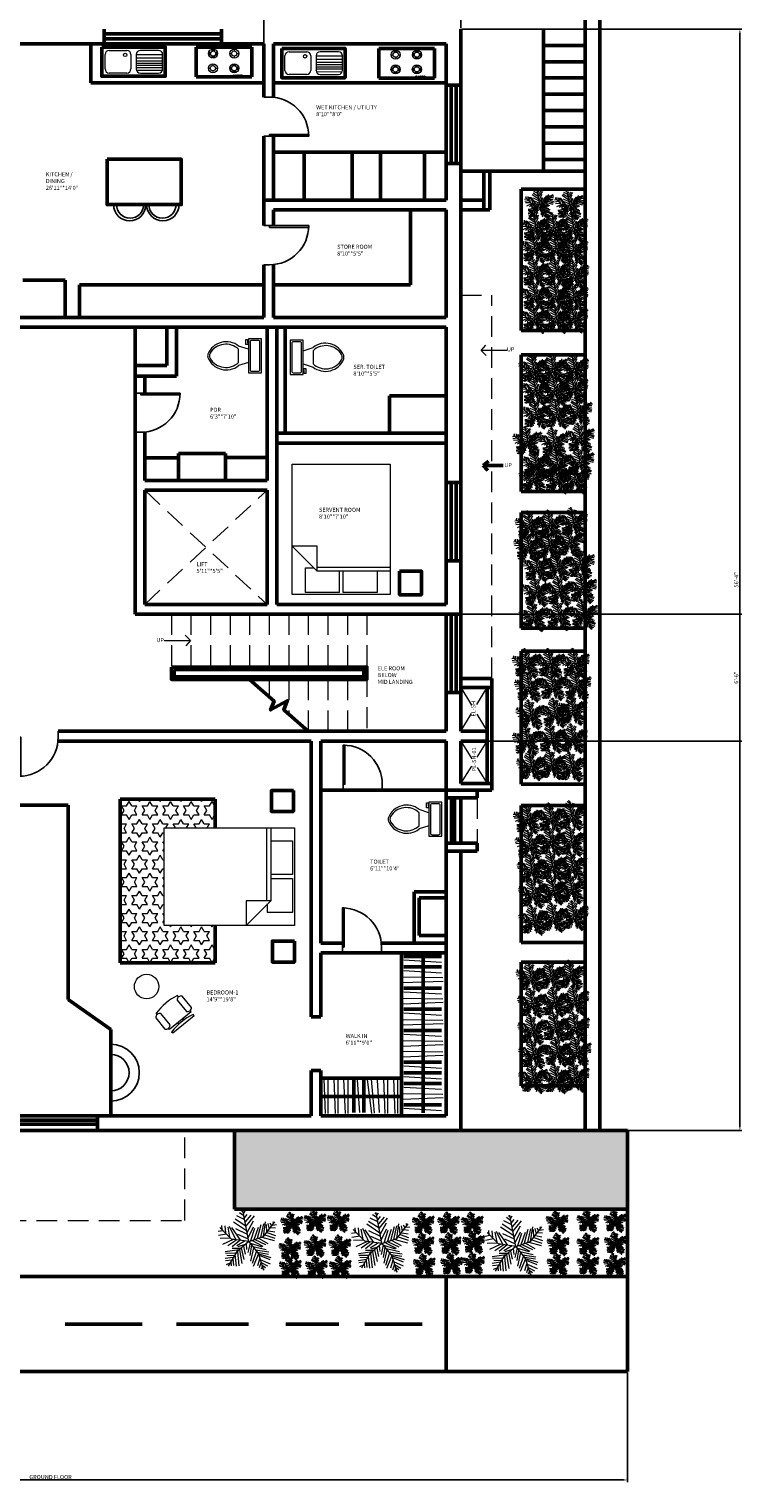
# Model space of a CAD drawing. Units: inches. Extents: x 5312 to 23584, y 2846 to 7447.
# Tile 3 of 12: x 9390 to 9827, y 2846 to 3738. Entities that reach past the tile are written whole.
import ezdxf

# ---------------------------------------------------------------- set-up
doc = ezdxf.new("R2010")
doc.units = ezdxf.units.IN
doc.linetypes.add('DASHED', pattern=[19.05, 12.7, -6.35])
for name, color, linetype, lineweight in [('A-ANNO-DIMS', 2, 'Continuous', 18), ('A-ANNO-TEXT', 3, 'Continuous', 18), ('A-AREA-IDEN', 7, 'Continuous', 18), ('A-DOOR', 4, 'Continuous', 25), ('A-FLOR-FIXT', 9, 'Continuous', 18), ('A-FLOR-OVHD', 8, 'DASHED', 18), ('A-FLOR-PATT', 252, 'Continuous', 13), ('A-FLOR-STRS', 3, 'Continuous', 18), ('A-FURN', 8, 'Continuous', 18), ('A-WALL', 7, 'Continuous', 50), ('L-PLNT', 82, 'Continuous', 13)]:
    doc.layers.add(name, color=color, linetype=linetype, lineweight=lineweight)
doc.styles.get("Standard").update_dxf_attribs({"font": 'arial.ttf'})
doc.dimstyles.new('ISO-25', dxfattribs={"dimtxt": 2.5, "dimasz": 2.5, "dimexe": 1.25, "dimexo": 0.625, "dimtad": 1, "dimlunit": 3, "dimtxsty": 'Standard', "dimcen": 2.5, "dimadec": 0, "dimazin": 0, "dimtfac": 1, "dimtmove": 0, "dimatfit": 3, "dimfxl": 1, "dimarcsym": 0})

# ---------------------------------------------------------------- blocks, each defined once
blk = doc.blocks.new('Toilet - top')
for p, q in [((-10, -8.5), (-8, -8.5)), ((-10, -9.5), (-10, -8.5)), ((-8, -8.5), (-8, -8)), ((-7, -8), (-7, -9.5)), ((-4, -8), (-6, -14)), ((4, -8), (6, -14)), ((9.5, -6), (9.5, -2)), ((-7, -9.5), (-10, -9.5)), ((4, -14), (-4, -14))]:
    blk.add_line(p, q)
blk.add_lwpolyline([(10.5, -8), (10.5, 0), (-10.5, 0), (-10.5, -8)], close=True)
for points in [[(-9.5, -2), (-9.5, -6)], [(8.5, -1), (-8.5, -1)], [(-8.5, -7), (8.5, -7)]]:
    blk.add_lwpolyline(points)
for centre, radius, start, end in [((-8.62, -1.88), 0.884, 81.8699, 188.1301), ((-8.62, -6.12), 0.884, 171.8699, 278.1301), ((8.62, -1.88), 0.884, 351.8699, 98.1301), ((8.62, -6.12), 0.884, 261.8699, 8.1301), ((3.52, -21.58), 12.17, 141.46911, 247.97143), ((4.2, -21.82), 11.33, 136.36773, 238.94682), ((-3.52, -21.58), 12.17, 292.02843, 38.53071), ((-4.2, -21.82), 11.33, 301.05301, 43.63209), ((0, -27.88), 4, 245.73182, 294.26817), ((0, -29), 4, 254.86053, 285.13947)]:
    blk.add_arc(centre, radius, start, end)
blk = doc.blocks.new('Bed - Queen')
for p, q in [((0, -80.00003), (0, 0)), ((0, 0), (59.99999, 0)), ((59.99999, 0), (59.99999, -80.00003)), ((7.99999, -1.2), (28.79998, -1.2)), ((7.99999, -14.4), (7.99999, -1.2)), ((28.79998, -1.2), (28.79998, -14.4)), ((31.19999, -1.2), (51.99999, -1.2)), ((31.19999, -14.4), (31.19999, -1.2)), ((51.99999, -1.2), (51.99999, -16.4)), ((0, -14.4), (44.8, -14.4)), ((44.8, -16.8), (0, -16.8)), ((59.99999, -29.6), (44.8, -14.4)), ((44.8, -14.4), (44.8, -29.6)), ((51.99999, -16.4), (46.79936, -16.4)), ((44.8, -29.6), (59.99999, -29.6)), ((59.99999, -80.00003), (0, -80.00003))]:
    blk.add_line(p, q)
blk = doc.blocks.new('Chair - Desk')
for p, q in [((-8.5, 0), (-8.5, -1)), ((-8.5, 0), (8.5, 0)), ((8.5, 0), (8.5, -1)), ((-10.5, -5), (-10.5, -14)), ((-8.5, -3), (-8.5, -4)), ((-8.5, -3), (8.5, -3)), ((-6.5, -14), (-6.5, -5)), ((-2, -3), (-2, -1.9355)), ((2, -1.9576), (2, -3)), ((6.5, -5), (6.5, -14)), ((8.5, -3), (8.5, -4)), ((10.5, -14), (10.5, -5)), ((-8.5, -15), (-8.5, -16)), ((8.5, -15), (8.5, -16))]:
    blk.add_line(p, q)
for centre, radius, start, end in [((-8.5, -6.5), 2.5, 36.8699, 143.1301), ((0, 34.625), 36.625, 256.5803, 283.4197), ((8.5, -6.5), 2.5, 36.8699, 143.1301), ((-8.5, -12.5), 2.5, 216.8699, 323.1301), ((0, 19.625), 36.625, 256.5803, 283.4197), ((8.5, -12.5), 2.5, 216.8699, 323.1301)]:
    blk.add_arc(centre, radius, start, end)
blk = doc.blocks.new('*U2')
for p, q in [((0, 0), (0, -6)), ((40, 0), (40, -6))]:
    blk.add_line(p, q)
blk.add_lwpolyline([(0, 0), (0, 40), (1.75, 40), (1.75, 0)], close=True)
blk.add_arc((0, 0), 40, 0, 90)
blk = doc.blocks.new('*U18')
for p, q in [((-10.186, 53.64), (-13.084, 55.962)), ((0, 0), (-10.5, 57)), ((-9.099, 51.782), (-6.563, 55.962)), ((-48.585, 21.131), (-49.309, 29.026)), ((-43.513, 28.561), (-42.427, 15.558)), ((-35.544, 28.097), (-24.314, 3.947)), ((-3.665, 19.273), (-27.574, 35.527)), ((-5.114, 28.097), (-24.676, 40.636)), ((-7.288, 39.707), (-21.778, 46.673)), ((-8.737, 47.138), (-17.069, 52.711)), ((-7.65, 43.423), (-2.578, 49.46)), ((-5.839, 35.992), (4.667, 48.067)), ((-5.114, 27.632), (10.463, 46.673)), ((-2.941, 16.486), (8.652, 37.85)), ((-1.129, 6.734), (9.014, 26.704)), ((16.259, 5.805), (23.142, 31.348)), ((22.055, 7.198), (27.489, 32.277)), ((27, 9), (48, 36)), ((27.127, 9.056), (31.112, 35.992)), ((31.836, 30.883), (32.561, 16.486)), ((35.096, 32.741), (37.27, 22.524)), ((38.719, 34.134), (41.979, 28.561)), ((43.791, 29.954), (51.036, 30.883)), ((44.153, 36.456), (45.239, 32.741)), ((-47.498, 19.737), (-55.83, 18.344)), ((-40.615, 13.7), (-55.105, 10.913)), ((-31.5, 4.5), (-52.5, 25.5)), ((-33.37, 6.269), (-52.207, 5.34)), ((-28.299, 3.483), (-47.86, -5.805)), ((-38.442, 26.239), (-34.819, 7.663)), ((-21.416, 3.018), (-38.079, -8.128)), ((0, 0), (-31.5, 4.5)), ((-14.533, 2.09), (-30.834, 25.31)), ((-15.982, 2.09), (-30.11, -9.521)), ((-24.314, 23.917), (-2.941, 13.7)), ((0, 0), (-22.5, -19.5)), ((-6.563, 1.161), (-21.416, -8.128)), ((-20.691, 13.7), (-1.129, 4.876)), ((0, 0), (27, 9)), ((0, 0), (18, -22.5)), ((3.942, 1.625), (11.187, 24.381)), ((6.478, 1.625), (26.04, -8.592)), ((10.101, 3.483), (17.708, 26.239)), ((11.187, 3.483), (30.749, -5.805)), ((18.07, 5.805), (35.096, -3.483)), ((24.229, 7.663), (46.688, 1.625)), ((29.662, 12.307), (48.137, 6.269)), ((33.285, 16.486), (48.862, 10.913)), ((36.183, 19.737), (48.137, 17.88)), ((40.53, 25.775), (48.862, 24.846)), ((-17.431, -15.094), (-42.789, -18.809)), ((-24.314, -21.596), (-42.427, -22.06)), ((-26.849, -26.24), (-40.253, -25.775)), ((-22.5, -19.5), (-37.5, -45)), ((-15.257, -12.772), (-30.11, -12.772)), ((-25.038, -23.918), (-22.865, -45.281)), ((-20.691, -18.345), (-17.793, -44.352)), ((-6.563, -5.805), (-19.967, -9.985)), ((-17.069, -15.094), (-12.721, -40.172)), ((-13.446, -11.378), (-8.737, -32.741)), ((-9.461, -8.592), (-6.201, -23.453)), ((-4.752, -3.483), (-3.665, -14.629)), ((2.493, -3.019), (-1.491, -20.202)), ((1.769, -2.555), (24.229, -9.521)), ((5.029, -6.27), (2.131, -25.775)), ((9.014, -11.378), (3.58, -35.992)), ((14.085, -16.951), (6.478, -40.172)), ((7.565, -9.056), (32.198, -14.629)), ((18.07, -22.524), (8.289, -45.745)), ((12.274, -15.094), (36.907, -18.809)), ((16.259, -19.738), (36.183, -22.989)), ((18, -22.5), (27, -52.5)), ((18.433, -22.524), (40.53, -29.026)), ((19.157, -25.311), (38.719, -33.206)), ((-28.299, -29.026), (-42.789, -31.348)), ((-30.834, -34.135), (-42.427, -35.528)), ((-34.457, -39.708), (-40.978, -42.494)), ((-32.646, -36.921), (-31.921, -44.352)), ((-29.023, -30.884), (-27.936, -43.887)), ((20.244, -30.419), (15.897, -44.816)), ((22.78, -37.85), (19.519, -48.532)), ((21.331, -32.741), (39.081, -40.636)), ((22.78, -38.314), (34.372, -44.816)), ((24.591, -45.745), (23.142, -50.854)), ((24.591, -43.423), (30.749, -47.603)), ((26.764, -49.925), (28.213, -50.854))]:
    blk.add_line(p, q)
blk = doc.blocks.new('WARDROBE-HANGER')
for p, q in [((0, 3.4), (24.8, 3.4)), ((0, 1.32), (24.99, 0))]:
    blk.add_line(p, q)
blk = doc.blocks.new('WARDROBE-HANGER-B')
for p, q in [((0, 21.08), (0.79, 0)), ((2.48, 21.08), (2.48, 0))]:
    blk.add_line(p, q)
blk = doc.blocks.new('STAIR-ARROW')
for p, q in [((0, 3.17), (16.03, 3.17)), ((16.03, 3.17), (12.89, 6.38)), ((16.03, 3.17), (13.15, 0))]:
    blk.add_line(p, q)
blk = doc.blocks.new('*D45')
at = {"layer": 'A-ANNO-DIMS', "color": 0, "lineweight": -2, "transparency": 16777216}
for p, q in [((8952.82, 2913.28), (8952.82, 2846.15)), ((9757.28, 2913.28), (9757.28, 2846.15)), ((8955.32, 2847.4), (9754.78, 2847.4))]:
    blk.add_line(p, q, dxfattribs=at)
at = {"layer": 'A-ANNO-DIMS', "color": 0, "transparency": 16777216}
for points in [[(8955.32, 2847.82), (8955.32, 2846.98), (8952.82, 2847.4)], [(9754.78, 2847.82), (9754.78, 2846.98), (9757.28, 2847.4)]]:
    blk.add_solid(points, dxfattribs=at)
at = {"layer": 'DEFPOINTS', "color": 0, "transparency": 16777216}
for p in [(8952.82, 2913.9), (9757.28, 2913.9), (9757.28, 2847.4)]:
    blk.add_point(p, dxfattribs=at)
at = {"layer": 'A-ANNO-DIMS', "color": 0, "transparency": 16777216, "insert": (9355.05, 2849.32), "char_height": 2.5, "attachment_point": 5}
blk.add_mtext('67\'-0 1/2"', dxfattribs=at)
blk = doc.blocks.new('*D48')
at = {"layer": 'A-ANNO-DIMS', "color": 0, "lineweight": -2, "transparency": 16777216}
for p, q in [((9021.01, 3738.27), (9021.01, 4212.68)), ((9023.51, 4211.43), (9652.51, 4211.43)), ((9655.01, 3738.27), (9655.01, 4212.68))]:
    blk.add_line(p, q, dxfattribs=at)
at = {"layer": 'A-ANNO-DIMS', "color": 0, "transparency": 16777216}
for points in [[(9023.51, 4211.85), (9023.51, 4211.01), (9021.01, 4211.43)], [(9652.51, 4211.85), (9652.51, 4211.01), (9655.01, 4211.43)]]:
    blk.add_solid(points, dxfattribs=at)
at = {"layer": 'DEFPOINTS', "color": 0, "transparency": 16777216}
for p in [(9655.01, 4211.43), (9021.01, 3737.65), (9655.01, 3737.65)]:
    blk.add_point(p, dxfattribs=at)
at = {"layer": 'A-ANNO-DIMS', "color": 0, "transparency": 16777216, "insert": (9338.01, 4213.33), "char_height": 2.5, "attachment_point": 5}
blk.add_mtext('52\'-10"', dxfattribs=at)
blk = doc.blocks.new('*D49')
at = {"layer": 'A-ANNO-DIMS', "color": 0, "lineweight": -2, "transparency": 16777216}
for p, q in [((9655.63, 3737.65), (9827.46, 3737.65)), ((9826.21, 3735.15), (9826.21, 3064.28)), ((9655.63, 3061.78), (9827.46, 3061.78))]:
    blk.add_line(p, q, dxfattribs=at)
at = {"layer": 'A-ANNO-DIMS', "color": 0, "transparency": 16777216}
for points in [[(9825.8, 3735.15), (9826.63, 3735.15), (9826.21, 3737.65)], [(9825.8, 3064.28), (9826.63, 3064.28), (9826.21, 3061.78)]]:
    blk.add_solid(points, dxfattribs=at)
at = {"layer": 'DEFPOINTS', "color": 0, "transparency": 16777216}
for p in [(9655.01, 3737.65), (9655.01, 3061.78), (9826.21, 3061.78)]:
    blk.add_point(p, dxfattribs=at)
at = {"layer": 'A-ANNO-DIMS', "color": 0, "transparency": 16777216, "insert": (9824.31, 3399.71), "char_height": 2.5, "attachment_point": 5, "rotation": 90}
blk.add_mtext('56\'-4"', dxfattribs=at)
blk = doc.blocks.new('*D55')
at = {"layer": 'A-ANNO-DIMS', "color": 0, "lineweight": -2, "transparency": 16777216}
for p, q in [((9205.01, 3729.27), (9205.01, 4212.68)), ((9207.51, 4211.43), (9531.51, 4211.43)), ((9534.01, 3705.2), (9534.01, 4212.68))]:
    blk.add_line(p, q, dxfattribs=at)
at = {"layer": 'A-ANNO-DIMS', "color": 0, "transparency": 16777216}
for points in [[(9207.51, 4211.85), (9207.51, 4211.01), (9205.01, 4211.43)], [(9531.51, 4211.85), (9531.51, 4211.01), (9534.01, 4211.43)]]:
    blk.add_solid(points, dxfattribs=at)
at = {"layer": 'DEFPOINTS', "color": 0, "transparency": 16777216}
for p in [(9534.01, 4211.43), (9205.01, 3728.65), (9534.01, 3704.57)]:
    blk.add_point(p, dxfattribs=at)
at = {"layer": 'A-ANNO-DIMS', "color": 0, "transparency": 16777216, "insert": (9369.51, 4213.33), "char_height": 2.5, "attachment_point": 5}
blk.add_mtext('27\'-5"', dxfattribs=at)
blk = doc.blocks.new('*D56')
at = {"layer": 'A-ANNO-DIMS', "color": 0, "lineweight": -2, "transparency": 16777216}
for p, q in [((9655.63, 3378.65), (9827.46, 3378.65)), ((9826.21, 3376.15), (9826.21, 3303.28)), ((9655.63, 3300.78), (9827.46, 3300.78))]:
    blk.add_line(p, q, dxfattribs=at)
at = {"layer": 'A-ANNO-DIMS', "color": 0, "transparency": 16777216}
for points in [[(9825.8, 3376.15), (9826.63, 3376.15), (9826.21, 3378.65)], [(9825.8, 3303.28), (9826.63, 3303.28), (9826.21, 3300.78)]]:
    blk.add_solid(points, dxfattribs=at)
at = {"layer": 'DEFPOINTS', "color": 0, "transparency": 16777216}
for p in [(9655.01, 3378.65), (9655.01, 3300.78), (9826.21, 3300.78)]:
    blk.add_point(p, dxfattribs=at)
at = {"layer": 'A-ANNO-DIMS', "color": 0, "transparency": 16777216, "insert": (9824.31, 3339.71), "char_height": 2.5, "attachment_point": 5, "rotation": 90}
blk.add_mtext('6\'-6"', dxfattribs=at)

msp = doc.modelspace()

# ---------------------------------------------------------------- hatches: boundary and pattern name
at = {"layer": 'A-FLOR-PATT'}
h = msp.add_hatch(dxfattribs=at)
h.set_pattern_fill('STARS', color=256)
h.set_pattern_definition([(0, (2182.2664, -374.049), (0, 5.4992613), [3.175, -3.175]), (60, (2182.2664, -374.049), (-4.7625, 2.7496307), [3.175, -3.175]), (120, (2183.854, -371.2995), (-4.7625, -2.7496307), [3.175, -3.175])])
h.paths.add_polyline_path([(9472.781, 3247.617), (9504.204, 3247.617), (9504.204, 3265.201), (9445.963, 3265.201), (9445.963, 3164.723), (9504.204, 3164.723), (9504.204, 3187.617), (9472.781, 3187.617)])
h = msp.add_hatch(dxfattribs=at)
h.set_pattern_fill('ANGLE', color=256)
h.set_pattern_definition([(0, (2182.2664, -374.049), (0, 6.985), [5.08, -1.905]), (90, (2182.2664, -374.049), (-6.985, 4e-16), [5.08, -1.905])])
h.paths.add_polyline_path([(9757.283, 3061.779), (9646.009, 3061.779), (9516.127, 3061.779), (9516.127, 3013.653), (9757.283, 3013.653)])
h.paths.add_polyline_path([(9030.009, 3030.646), (9021.009, 3030.646), (8952.82, 3030.646), (8952.82, 3007.004), (9030.009, 3007.004)])

# ---------------------------------------------------------------- linework, layer by layer
at = {"layer": 'A-DOOR'}
for centre, radius, start, end in [((9451.679, 3629.961), 9.935, 180, 0), ((9451.945, 3629.961), 8.375, 180, 0), ((9472.075, 3629.961), 9.948, 180, 0), ((9471.776, 3629.961), 8.375, 180, 0), ((9440.091, 3097.323), 17.484, 270, 90), ((9440.091, 3097.323), 17.484, 270, 90), ((9440.091, 3097.323), 11.255, 270, 90)]:
    msp.add_arc(centre, radius, start, end, dxfattribs=at)
at = {"layer": 'A-FLOR-FIXT'}
for p, q in [((9436.608, 3713.16), (9436.608, 3722.083)), ((9439.108, 3724.583), (9449.959, 3724.583)), ((9452.459, 3722.083), (9452.459, 3713.16)), ((9455.758, 3722.083), (9455.758, 3713.16)), ((9455.758, 3722.083), (9471.946, 3722.083)), ((9455.758, 3720.061), (9471.946, 3720.061)), ((9469.446, 3724.583), (9458.258, 3724.583)), ((9471.946, 3713.16), (9471.946, 3722.083)), ((9513.105, 3722.627), (9514.279, 3722.627)), ((9515.882, 3725.404), (9515.882, 3724.249)), ((9515.882, 3721.043), (9515.882, 3719.85)), ((9517.484, 3722.627), (9518.658, 3722.627)), ((9546.988, 3712.322), (9546.988, 3721.245)), ((9549.488, 3723.745), (9560.339, 3723.745)), ((9562.839, 3721.245), (9562.839, 3712.322)), ((9566.137, 3721.245), (9566.137, 3712.322)), ((9566.137, 3721.245), (9582.325, 3721.245)), ((9579.825, 3723.745), (9568.637, 3723.745)), ((9582.325, 3712.322), (9582.325, 3721.245)), ((9612.215, 3721.924), (9612.204, 3721.924)), ((9612.204, 3721.924), (9613.389, 3721.924)), ((9614.992, 3720.321), (9614.992, 3719.148)), ((9616.595, 3721.924), (9617.769, 3721.924)), ((9455.758, 3718.237), (9471.946, 3718.237)), ((9455.758, 3716.659), (9471.946, 3716.659)), ((9455.758, 3715.403), (9471.946, 3715.403)), ((9455.758, 3714.107), (9455.758, 3714.107)), ((9455.758, 3714.107), (9471.946, 3714.107)), ((9455.758, 3713.16), (9455.758, 3713.328)), ((9455.907, 3712.348), (9471.82, 3712.378)), ((9499.993, 3713.609), (9501.167, 3713.609)), ((9502.77, 3716.386), (9502.77, 3715.212)), ((9502.77, 3712.006), (9502.77, 3710.833)), ((9504.373, 3713.609), (9505.547, 3713.609)), ((9566.137, 3719.223), (9582.325, 3719.223)), ((9566.137, 3717.398), (9582.325, 3717.398)), ((9566.137, 3715.82), (9582.325, 3715.82)), ((9566.137, 3714.565), (9582.325, 3714.565)), ((9566.137, 3713.269), (9566.137, 3713.269)), ((9566.137, 3713.269), (9582.325, 3713.269)), ((9566.137, 3712.322), (9566.137, 3712.489)), ((9566.287, 3711.51), (9582.2, 3711.539)), ((9449.959, 3710.66), (9439.108, 3710.66)), ((9458.258, 3710.66), (9469.446, 3710.66)), ((9560.339, 3709.822), (9549.488, 3709.822)), ((9568.637, 3709.822), (9579.825, 3709.822))]:
    msp.add_line(p, q, dxfattribs=at)
for centre, radius in [((9515.882, 3722.627), 2.777), ((9515.882, 3722.646), 1.603), ((9614.992, 3721.924), 2.777), ((9614.992, 3721.924), 1.603), ((9502.77, 3713.609), 2.777), ((9502.77, 3713.609), 1.603)]:
    msp.add_circle(centre, radius, dxfattribs=at)
for centre, start, end in [((9439.108, 3722.083), 90, 180), ((9449.959, 3722.083), 0, 90), ((9458.258, 3722.083), 90, 180), ((9469.446, 3722.083), 0, 90), ((9549.488, 3721.245), 90, 180), ((9560.339, 3721.245), 0, 90), ((9568.637, 3721.245), 90, 180), ((9579.825, 3721.245), 0, 90), ((9439.108, 3713.16), 180, 270), ((9449.959, 3713.16), 270, 0), ((9458.258, 3713.16), 180, 270), ((9469.446, 3713.16), 270, 0), ((9549.488, 3712.322), 180, 270), ((9560.339, 3712.322), 270, 0), ((9568.637, 3712.322), 180, 270), ((9579.825, 3712.322), 270, 0)]:
    msp.add_arc(centre, 2.5, start, end, dxfattribs=at)
at = {"layer": 'A-FLOR-OVHD'}
for p, q in [((9655.009, 3574.399), (9673.869, 3574.399)), ((9673.869, 3339.256), (9673.869, 3574.399)), ((9461.009, 3454.646), (9536.009, 3384.646)), ((9461.009, 3384.646), (9536.009, 3454.646)), ((9477.315, 3378.646), (9477.315, 3338.606)), ((9489.315, 3378.646), (9489.315, 3346.136)), ((9501.315, 3378.646), (9501.315, 3346.136)), ((9513.315, 3378.646), (9513.315, 3346.136)), ((9525.315, 3378.646), (9525.315, 3346.136)), ((9537.315, 3378.646), (9537.315, 3346.136)), ((9549.315, 3378.646), (9549.315, 3346.136)), ((9561.315, 3378.646), (9561.315, 3346.136)), ((9573.315, 3378.646), (9573.315, 3346.136)), ((9585.315, 3378.646), (9585.315, 3346.136)), ((9597.315, 3378.646), (9597.315, 3306.779)), ((9537.315, 3338.606), (9537.315, 3327.997)), ((9549.315, 3338.606), (9549.315, 3317.388)), ((9561.315, 3338.606), (9561.315, 3306.779)), ((9573.315, 3338.606), (9573.315, 3306.779)), ((9585.315, 3338.606), (9585.315, 3306.779)), ((9655.009, 3333.708), (9671.048, 3306.779)), ((9655.009, 3306.779), (9671.048, 3333.708)), ((9655.009, 3300.779), (9671.048, 3274.653)), ((9655.009, 3274.653), (9671.048, 3300.779)), ((9671.048, 3306.779), (9671.048, 3306.779)), ((9665.054, 3265.866), (9665.054, 3238.12)), ((9485.603, 3006.697), (9485.603, 3061.779)), ((9127.897, 3006.697), (9485.603, 3006.697))]:
    msp.add_line(p, q, dxfattribs=at)
at = {"layer": 'A-FURN'}
for p, q in [((9620.002, 3166.502), (9643.154, 3165.13)), ((9620.002, 3160.001), (9643.154, 3158.629)), ((9620.002, 3147), (9643.154, 3145.627)), ((9620.002, 3133.998), (9643.154, 3132.626)), ((9620.002, 3120.997), (9643.154, 3119.624)), ((9620.002, 3101.495), (9643.154, 3100.122)), ((9591.382, 3092.714), (9592.659, 3072.858)), ((9603.585, 3092.714), (9604.862, 3072.858)), ((9620.002, 3094.994), (9643.154, 3093.622)), ((9620.002, 3088.493), (9643.154, 3087.121)), ((9620.002, 3075.492), (9643.154, 3074.119))]:
    msp.add_line(p, q, dxfattribs=at)
for centre, radius in [((9448.939, 3721.761), 1.035), ((9502.901, 3722.646), 2.777), ((9502.901, 3722.646), 1.603), ((9559.318, 3720.922), 1.035), ((9627.973, 3721.905), 2.777), ((9627.973, 3721.924), 1.603), ((9515.857, 3713.637), 2.777), ((9515.857, 3713.637), 1.603), ((9614.861, 3712.887), 2.777), ((9614.861, 3712.887), 1.603), ((9627.948, 3712.915), 2.777), ((9627.948, 3712.915), 1.603), ((9515.611, 3709.213), 0.395), ((9516.925, 3709.156), 0.395), ((9518.186, 3709.19), 0.395), ((9519.385, 3709.196), 0.395), ((9520.555, 3709.21), 0.395), ((9627.702, 3708.491), 0.395), ((9629.016, 3708.434), 0.395), ((9630.277, 3708.468), 0.395), ((9631.476, 3708.474), 0.395), ((9632.646, 3708.488), 0.395), ((9462.096, 3150.15), 7.51)]:
    msp.add_circle(centre, radius, dxfattribs=at)
at = {"layer": 'A-WALL'}
for p, q in [((9740.323, 3061.779), (9740.323, 4009.837)), ((9731.323, 3061.779), (9731.323, 4000.837)), ((9436.116, 3728.646), (9436.116, 3737.646)), ((9436.116, 3734.646), (9508.116, 3734.646)), ((9508.116, 3731.646), (9436.116, 3731.646)), ((9508.116, 3737.646), (9508.116, 3728.646)), ((9655.009, 3737.646), (9655.009, 3554.646)), ((9705.72, 3737.646), (9705.72, 3650.559)), ((9534.009, 3728.646), (9211.009, 3728.646)), ((9427.949, 3704.571), (9427.949, 3728.646)), ((9508.116, 3728.646), (9436.116, 3728.646)), ((9492.456, 3726.447), (9492.456, 3708.298)), ((9526.608, 3726.447), (9492.456, 3726.447)), ((9500.124, 3722.646), (9500.113, 3722.646)), ((9500.113, 3722.646), (9501.298, 3722.646)), ((9502.901, 3725.423), (9502.901, 3724.249)), ((9502.901, 3721.043), (9502.901, 3719.87)), ((9504.504, 3722.646), (9505.678, 3722.646)), ((9526.608, 3708.298), (9526.608, 3726.447)), ((9534.009, 3728.646), (9534.009, 3695.928)), ((9540.009, 3728.646), (9540.009, 3695.808)), ((9646.009, 3728.646), (9540.009, 3728.646)), ((9604.547, 3725.725), (9604.547, 3707.576)), ((9638.699, 3725.725), (9604.547, 3725.725)), ((9614.992, 3724.701), (9614.992, 3723.527)), ((9625.196, 3721.905), (9625.196, 3721.905)), ((9625.196, 3721.905), (9626.37, 3721.905)), ((9627.973, 3724.682), (9627.973, 3723.527)), ((9627.973, 3720.321), (9627.973, 3719.128)), ((9629.576, 3721.905), (9630.75, 3721.905)), ((9638.699, 3707.576), (9638.699, 3725.725)), ((9646.009, 3728.646), (9646.009, 3632.646)), ((9705.72, 3727.646), (9731.323, 3727.646)), ((9513.08, 3713.637), (9514.254, 3713.637)), ((9515.857, 3716.414), (9515.857, 3715.24)), ((9515.857, 3712.034), (9515.857, 3710.86)), ((9517.46, 3713.637), (9518.634, 3713.637)), ((9612.084, 3712.887), (9613.258, 3712.887)), ((9614.861, 3715.664), (9614.861, 3714.49)), ((9614.861, 3711.284), (9614.861, 3710.11)), ((9616.464, 3712.887), (9617.638, 3712.887)), ((9625.172, 3712.915), (9626.345, 3712.915)), ((9627.948, 3715.692), (9627.948, 3714.518)), ((9627.948, 3711.312), (9627.948, 3710.138)), ((9629.551, 3712.915), (9630.725, 3712.915)), ((9705.72, 3717.646), (9731.323, 3717.646)), ((9534.009, 3704.571), (9427.949, 3704.571)), ((9492.456, 3708.298), (9526.608, 3708.298)), ((9540.009, 3704.571), (9540.009, 3704.571)), ((9540.009, 3704.571), (9646.009, 3704.571)), ((9604.547, 3707.576), (9638.699, 3707.576)), ((9646.009, 3655.161), (9646.009, 3703.161)), ((9646.009, 3703.161), (9655.009, 3703.161)), ((9649.009, 3655.161), (9649.009, 3703.161)), ((9652.009, 3703.161), (9652.009, 3655.161)), ((9655.009, 3703.161), (9655.009, 3655.161)), ((9705.72, 3707.646), (9731.323, 3707.646)), ((9705.72, 3697.646), (9731.323, 3697.646)), ((9705.72, 3687.646), (9731.323, 3687.646)), ((9705.72, 3677.646), (9731.323, 3677.646)), ((9534.009, 3671.928), (9534.009, 3626.646)), ((9540.009, 3672.978), (9540.009, 3632.646)), ((9705.72, 3667.646), (9731.323, 3667.646)), ((9540.009, 3662.2), (9646.009, 3662.2)), ((9705.72, 3657.646), (9731.323, 3657.646)), ((9655.009, 3655.161), (9646.009, 3655.161)), ((9731.323, 3650.559), (9655.009, 3650.559)), ((9669.132, 3632.646), (9669.132, 3650.559)), ((9672.838, 3626.646), (9672.838, 3650.559)), ((9646.009, 3632.646), (9534.009, 3632.646)), ((9655.009, 3632.646), (9669.132, 3632.646)), ((9669.132, 3632.646), (9669.132, 3626.646)), ((9731.323, 3639.466), (9692.046, 3639.466)), ((9692.046, 3639.466), (9692.046, 3552.709)), ((9534.009, 3626.646), (9534.009, 3617.023)), ((9646.009, 3626.646), (9540.009, 3626.646)), ((9540.009, 3626.646), (9540.009, 3617.023)), ((9624.059, 3580.732), (9624.059, 3626.646)), ((9646.009, 3626.646), (9646.009, 3560.646)), ((9669.132, 3626.646), (9655.009, 3626.646)), ((9669.132, 3626.646), (9672.838, 3626.646)), ((9534.009, 3593.023), (9534.009, 3585.878)), ((9540.009, 3585.878), (9540.008, 3593.143)), ((9386.03, 3583.618), (9412.168, 3583.618)), ((9412.168, 3583.618), (9412.168, 3560.646)), ((9420.858, 3577.967), (9420.858, 3580.732)), ((9420.858, 3580.732), (9534.009, 3580.732)), ((9420.858, 3560.646), (9420.858, 3577.967)), ((9534.009, 3585.878), (9534.009, 3560.646)), ((9540.009, 3585.878), (9540.009, 3560.646)), ((9540.009, 3580.732), (9624.059, 3580.732)), ((9534.009, 3560.646), (9377.388, 3560.646)), ((9540.009, 3560.646), (9646.009, 3560.646)), ((9540.009, 3554.646), (9377.388, 3554.646)), ((9455.009, 3554.646), (9455.009, 3378.646)), ((9474.406, 3531.221), (9474.406, 3554.646)), ((9480.406, 3524.692), (9480.406, 3554.646)), ((9536.009, 3554.646), (9536.009, 3460.646)), ((9540.009, 3554.646), (9646.009, 3554.646)), ((9542.009, 3554.646), (9542.009, 3384.646)), ((9547.186, 3489.646), (9547.186, 3554.646)), ((9646.009, 3554.646), (9646.009, 3384.646)), ((9655.009, 3554.646), (9655.009, 3554.646)), ((9655.009, 3554.646), (9655.009, 3378.646)), ((9692.046, 3552.709), (9731.323, 3552.709)), ((9692.046, 3537.705), (9731.323, 3537.705)), ((9692.046, 3537.705), (9692.046, 3453.961)), ((9474.406, 3531.221), (9455.009, 3531.221)), ((9455.009, 3524.692), (9480.406, 3524.692)), ((9461.009, 3524.692), (9461.009, 3513.194)), ((9646.009, 3512.616), (9611.082, 3512.616)), ((9611.082, 3512.616), (9611.082, 3489.646)), ((9461.009, 3490.362), (9461.009, 3460.646)), ((9542.009, 3489.646), (9646.009, 3489.646)), ((9542.009, 3483.646), (9646.009, 3483.646)), ((9481.715, 3474.489), (9461.009, 3474.489)), ((9481.715, 3460.646), (9481.715, 3477.326)), ((9481.715, 3477.326), (9510.537, 3477.326)), ((9510.537, 3477.326), (9510.537, 3460.646)), ((9510.537, 3474.808), (9536.009, 3474.808)), ((9668.6, 3469.857), (9671.917, 3472.579)), ((9668.6, 3469.857), (9680.993, 3469.857)), ((9668.6, 3469.857), (9671.487, 3466.827)), ((9536.009, 3460.646), (9461.009, 3460.646)), ((9536.009, 3454.646), (9461.009, 3454.646)), ((9461.009, 3454.646), (9461.009, 3384.646)), ((9536.009, 3454.646), (9536.009, 3384.646)), ((9646.009, 3411.4), (9646.009, 3459.4)), ((9646.009, 3459.4), (9655.009, 3459.4)), ((9649.009, 3411.4), (9649.009, 3459.4)), ((9652.009, 3459.4), (9652.009, 3411.4)), ((9655.009, 3459.4), (9655.009, 3411.4)), ((9692.046, 3453.961), (9731.323, 3453.961)), ((9692.046, 3441.04), (9731.323, 3441.04)), ((9692.046, 3441.04), (9692.046, 3370.139)), ((9655.009, 3411.4), (9646.009, 3411.4)), ((9461.009, 3384.646), (9536.009, 3384.646)), ((9542.009, 3384.646), (9646.009, 3384.646)), ((9455.009, 3378.646), (9542.009, 3378.646)), ((9655.009, 3378.646), (9542.009, 3378.646)), ((9646.009, 3378.646), (9646.009, 3306.779)), ((9646.009, 3330.646), (9646.009, 3378.646)), ((9646.009, 3378.646), (9655.009, 3378.646)), ((9649.009, 3330.646), (9649.009, 3378.646)), ((9652.009, 3378.646), (9652.009, 3330.646)), ((9655.009, 3378.646), (9655.009, 3306.779)), ((9655.009, 3378.646), (9655.009, 3330.646)), ((9692.046, 3370.139), (9731.323, 3370.139)), ((9692.046, 3356.023), (9731.323, 3356.023)), ((9692.046, 3356.023), (9692.046, 3274.362)), ((9525.315, 3338.606), (9540.319, 3325.342)), ((9671.048, 3339.256), (9655.009, 3339.256)), ((9671.048, 3339.256), (9673.869, 3339.256)), ((9673.869, 3339.256), (9673.869, 3270.68)), ((9655.009, 3330.646), (9646.009, 3330.646)), ((9655.009, 3333.708), (9673.869, 3333.708)), ((9671.048, 3333.708), (9671.048, 3306.779)), ((9546.312, 3320.043), (9561.315, 3306.779)), ((9407.712, 3300.779), (9563.009, 3300.779)), ((9407.833, 3306.779), (9646.009, 3306.779)), ((9563.009, 3300.779), (9563.009, 3131.674)), ((9569.009, 3300.779), (9569.009, 3176.779)), ((9569.009, 3300.779), (9646.009, 3300.779)), ((9646.009, 3300.779), (9646.009, 3070.779)), ((9671.048, 3306.779), (9655.009, 3306.779)), ((9655.009, 3300.779), (9671.048, 3300.779)), ((9655.009, 3300.779), (9655.009, 3274.653)), ((9671.048, 3300.779), (9671.048, 3306.779)), ((9671.048, 3300.779), (9671.048, 3274.653)), ((9673.869, 3274.653), (9655.009, 3274.653)), ((9692.046, 3274.362), (9731.323, 3274.362)), ((9504.204, 3265.201), (9445.963, 3265.201)), ((9445.963, 3265.201), (9445.963, 3164.723)), ((9504.204, 3247.617), (9504.204, 3265.201)), ((9569.009, 3270.68), (9646.009, 3270.68)), ((9646.009, 3270.68), (9646.009, 3270.68)), ((9646.009, 3270.68), (9665.054, 3270.68)), ((9665.054, 3265.866), (9646.009, 3265.866)), ((9649.246, 3265.866), (9649.246, 3265.866)), ((9649.246, 3265.866), (9649.246, 3238.12)), ((9651.153, 3265.866), (9651.153, 3265.716)), ((9651.153, 3265.716), (9651.153, 3238.12)), ((9655.009, 3265.866), (9655.009, 3238.12)), ((9665.054, 3270.68), (9665.054, 3265.866)), ((9665.054, 3270.68), (9671.048, 3270.68)), ((9673.869, 3270.68), (9671.048, 3270.68)), ((9375.565, 3261.354), (9413.869, 3261.354)), ((9413.869, 3261.354), (9413.869, 3142.191)), ((9692.046, 3261.248), (9731.323, 3261.248)), ((9692.046, 3261.248), (9692.046, 3177.116)), ((9665.054, 3238.12), (9646.009, 3238.12)), ((9646.009, 3233.2), (9665.054, 3233.2)), ((9655.009, 3233.2), (9655.009, 3061.779)), ((9665.054, 3233.2), (9665.054, 3238.12)), ((9626.202, 3176.779), (9626.202, 3208.299)), ((9626.202, 3208.299), (9646.009, 3208.299)), ((9646.009, 3204.617), (9629.416, 3204.617)), ((9629.416, 3204.617), (9629.416, 3181.501)), ((9504.204, 3164.723), (9504.204, 3187.617)), ((9569.009, 3176.779), (9583.292, 3176.779)), ((9606.122, 3176.779), (9646.009, 3176.779)), ((9629.416, 3181.501), (9646.009, 3181.501)), ((9692.046, 3177.116), (9731.323, 3177.116)), ((9569.009, 3170.779), (9646.009, 3170.779)), ((9569.009, 3170.779), (9569.009, 3131.674)), ((9618.471, 3093.959), (9618.471, 3170.779)), ((9620.002, 3168.691), (9643.154, 3168.691)), ((9631.731, 3169.764), (9631.731, 3072.569)), ((9445.963, 3164.723), (9504.204, 3164.723)), ((9620.002, 3162.19), (9643.154, 3162.19)), ((9692.046, 3165.135), (9731.323, 3165.135)), ((9692.046, 3165.135), (9692.046, 3089.247)), ((9620.002, 3149.189), (9643.154, 3149.189)), ((9413.869, 3142.191), (9440.091, 3123.866)), ((9563.009, 3131.674), (9569.009, 3131.674)), ((9620.002, 3136.187), (9643.154, 3136.187)), ((9440.091, 3123.866), (9440.091, 3070.779)), ((9620.002, 3123.186), (9643.154, 3123.186)), ((9563.009, 3098.558), (9563.009, 3098.558)), ((9563.009, 3098.558), (9569.009, 3098.558)), ((9563.009, 3098.558), (9563.009, 3070.779)), ((9569.009, 3098.558), (9569.009, 3070.779)), ((9620.002, 3103.684), (9643.154, 3103.684)), ((9620.002, 3097.183), (9643.154, 3097.183)), ((9569.009, 3093.959), (9618.471, 3093.959)), ((9589.218, 3092.714), (9589.218, 3072.858)), ((9595.319, 3092.714), (9595.319, 3072.858)), ((9618.471, 3093.959), (9618.471, 3070.779)), ((9620.002, 3090.682), (9643.154, 3090.682)), ((9692.046, 3089.247), (9731.323, 3089.247)), ((9569.834, 3082.786), (9617.526, 3082.786)), ((9620.002, 3077.681), (9643.154, 3077.681)), ((9375.565, 3070.779), (9563.009, 3070.779)), ((9431.962, 3070.779), (9431.962, 3061.779)), ((9569.009, 3070.779), (9646.009, 3070.779)), ((9369.565, 3061.779), (9646.009, 3061.779)), ((9372.219, 3065.688), (9431.962, 3065.688)), ((9373.71, 3068.089), (9431.962, 3068.089)), ((9431.962, 3065.688), (9431.962, 3065.688)), ((9516.127, 3061.779), (9516.127, 3061.779)), ((9516.127, 3061.779), (9516.127, 3013.653)), ((9757.283, 3061.779), (9646.009, 3061.779)), ((9757.283, 2913.9), (9757.283, 3061.779)), ((9516.127, 3013.653), (9757.283, 3013.653)), ((8952.82, 2972.273), (9757.283, 2972.273)), ((9646.009, 2972.273), (9646.009, 2913.9)), ((9412.184, 2943.087), (9459.269, 2943.087)), ((9480.528, 2943.087), (9524.604, 2943.087)), ((9547.44, 2943.087), (9580.054, 2943.087)), ((9596.053, 2943.087), (9631.138, 2943.087)), ((8952.82, 2913.9), (9757.283, 2913.9))]:
    msp.add_line(p, q, dxfattribs=at)
for points in [[(9434.608, 3726.583), (9473.512, 3726.583), (9473.512, 3708.66), (9434.608, 3708.66)], [(9544.988, 3725.745), (9583.892, 3725.745), (9583.892, 3707.822), (9544.988, 3707.822)], [(9437.808, 3657.792), (9483.37, 3657.792), (9483.37, 3629.961), (9437.808, 3629.961)], [(9558.714, 3662.2), (9588.194, 3662.2), (9588.194, 3632.646), (9558.714, 3632.646)], [(9605.674, 3662.2), (9632.712, 3662.2), (9632.712, 3632.646), (9605.674, 3632.646)], [(9617.375, 3405.094), (9630.776, 3405.094), (9630.776, 3390.596), (9617.375, 3390.596)], [(9477.315, 3346.136), (9597.315, 3346.136), (9597.315, 3338.606), (9477.315, 3338.606)], [(9479.054, 3344.698), (9595.323, 3344.698), (9595.323, 3340.135), (9479.054, 3340.135)], [(9552.166, 3270.444), (9538.721, 3270.444), (9538.721, 3257.633), (9552.166, 3257.633)], [(9552.781, 3178.027), (9539.337, 3178.027), (9539.337, 3165.215), (9552.781, 3165.215)]]:
    msp.add_lwpolyline(points, close=True, dxfattribs=at)
msp.add_lwpolyline([(9539.863, 3325.745), (9540.319, 3325.342), (9538.177, 3319.901), (9548.453, 3325.485), (9546.312, 3320.043), (9550.252, 3316.56)], dxfattribs=at)

# ---------------------------------------------------------------- block references
at = {"layer": 'A-DOOR', "yscale": 0.6, "zscale": 0.6}
for p, xscale, rotation in [((9537.609, 3671.928), -0.6, 270), ((9537.609, 3617.023), 0.6, 270), ((9458.632, 3514.244), 0.6, 270), ((9383.833, 3303.179), -0.6, 180)]:
    msp.add_blockref('*U2', p, dxfattribs=dict(at, xscale=xscale, rotation=rotation))
at = {"layer": 'A-DOOR', "xscale": 0.6, "yscale": 0.6, "zscale": 0.6}
for p in [(9582.766, 3274.28), (9582.242, 3174.379)]:
    msp.add_blockref('*U2', p, dxfattribs=at)
at = {"layer": 'A-FLOR-FIXT'}
for p, rotation in [((9532.558, 3537.158), 270), ((9550.228, 3536.281), 90), ((9643.323, 3252.832), 270)]:
    msp.add_blockref('Toilet - top', p, dxfattribs=dict(at, rotation=rotation))
at = {"layer": 'A-FLOR-STRS'}
for p, rotation in [((9683.461, 3543.632), 179.8030510924859), ((9472.972, 3359.231), 0.2298133556746135)]:
    msp.add_blockref('STAIR-ARROW', p, dxfattribs=dict(at, rotation=rotation))
at = {"layer": 'A-FURN'}
for name, p, rotation in [('Bed - Queen', (9611.527, 3390.694), 180), ('Bed - Queen', (9552.781, 3247.617), 269.9999999999999), ('WARDROBE-HANGER', (9643.943, 3156.742), 182.1189074632503), ('Chair - Desk', (9484.671, 3126.847), 219.2765593068386), ('WARDROBE-HANGER', (9643.943, 3143.74), 182.1189074632546), ('WARDROBE-HANGER', (9643.943, 3130.739), 182.1189074632526), ('WARDROBE-HANGER', (9643.943, 3117.738), 182.1189074632526), ('WARDROBE-HANGER', (9643.943, 3111.237), 182.1189074632526), ('WARDROBE-HANGER-B', (9570.929, 3072.238), 0.277717142694316), ('WARDROBE-HANGER-B', (9577.031, 3072.238), 0.2777171426851295), ('WARDROBE-HANGER-B', (9583.132, 3072.238), 0.2777171426851295), ('WARDROBE-HANGER-B', (9599.301, 3072.158), 5.221751322829238), ('WARDROBE-HANGER-B', (9607.539, 3072.238), 0.2777171426733181), ('WARDROBE-HANGER-B', (9613.64, 3072.238), 0.2777171426733181), ('WARDROBE-HANGER', (9643.943, 3085.234), 182.1189074632546)]:
    msp.add_blockref(name, p, dxfattribs=dict(at, rotation=rotation))
at = {"layer": 'L-PLNT'}
for p, xscale, yscale, zscale in [((9703.448, 3630.026), 0.169248058745953, 0.169248058745953, 0.169248058745953), ((9721.815, 3629.497), 0.169248058745953, 0.169248058745953, 0.169248058745953), ((9701.1, 3615.532), 0.169248058745953, 0.169248058745953, 0.169248058745953), ((9712.5, 3615.532), 0.169248058745953, 0.169248058745953, 0.169248058745953), ((9724.356, 3615.532), 0.169248058745953, 0.169248058745953, 0.169248058745953), ((9700.644, 3602.775), 0.169248058745953, 0.169248058745953, 0.169248058745953), ((9713.754, 3602.775), 0.169248058745953, 0.169248058745953, 0.169248058745953), ((9724.47, 3601.517), 0.169248058745953, 0.169248058745953, 0.169248058745953), ((9700.716, 3587.977), 0.169248058745953, 0.169248058745953, 0.169248058745953), ((9713.873, 3587.977), 0.169248058745953, 0.169248058745953, 0.169248058745953), ((9724.971, 3586.605), 0.169248058745953, 0.169248058745953, 0.169248058745953), ((9700.819, 3573.567), 0.169248058745953, 0.169248058745953, 0.169248058745953), ((9713.724, 3573.567), 0.169248058745953, 0.169248058745953, 0.169248058745953), ((9724.67, 3572.992), 0.169248058745953, 0.169248058745953, 0.169248058745953), ((9700.708, 3559.625), 0.169248058745953, 0.169248058745953, 0.169248058745953), ((9713.957, 3559.625), 0.169248058745953, 0.169248058745953, 0.169248058745953), ((9724.513, 3559.94), 0.169248058745953, 0.169248058745953, 0.169248058745953), ((9699.835, 3529.007), 0.169248058745953, 0.169248058745953, 0.169248058745953), ((9711.766, 3529.125), 0.169248058745953, 0.169248058745953, 0.169248058745953), ((9724.878, 3529.125), 0.169248058745953, 0.169248058745953, 0.169248058745953), ((9701.017, 3515.552), 0.169248058745953, 0.169248058745953, 0.169248058745953), ((9713.065, 3515.552), 0.169248058745953, 0.169248058745953, 0.169248058745953), ((9724.523, 3516.85), 0.169248058745953, 0.169248058745953, 0.169248058745953), ((9701.479, 3501.002), 0.169248058745953, 0.169248058745953, 0.169248058745953), ((9714.324, 3501.101), 0.169248058745953, 0.169248058745953, 0.169248058745953), ((9727.086, 3502.535), 0.169248058745953, 0.169248058745953, 0.169248058745953), ((9696.205, 3484.392), 0.169248058745953, 0.169248058745953, 0.169248058745953), ((9712.493, 3483.627), 0.169248058745953, 0.169248058745953, 0.169248058745953), ((9728.434, 3486.306), 0.169248058745953, 0.169248058745953, 0.169248058745953), ((9701.321, 3470.483), 0.169248058745953, 0.169248058745953, 0.169248058745953), ((9714.54, 3470.483), 0.169248058745953, 0.169248058745953, 0.169248058745953), ((9728.248, 3471.583), 0.169248058745953, 0.169248058745953, 0.169248058745953), ((9700.066, 3461.695), 0.169248058745953, 0.169248058745953, 0.169248058745953), ((9714.575, 3461.219), 0.169248058745953, 0.169248058745953, 0.169248058745953), ((9725.375, 3461.243), 0.169248058745953, 0.169248058745953, 0.169248058745953), ((9724.211, 3434.594), 0.169248058745953, 0.169248058745953, 0.169248058745953), ((9697.623, 3432.6), 0.169248058745953, 0.169248058745953, 0.169248058745953), ((9709.999, 3432.999), 0.169248058745953, 0.169248058745953, 0.169248058745953), ((9696.815, 3419.749), 0.169248058745953, 0.169248058745953, 0.169248058745953), ((9709.477, 3420.505), 0.169248058745953, 0.169248058745953, 0.169248058745953), ((9722.038, 3422.269), 0.169248058745953, 0.169248058745953, 0.169248058745953), ((9702.06, 3407.194), 0.169248058745953, 0.169248058745953, 0.169248058745953), ((9714.704, 3407.806), 0.169248058745953, 0.169248058745953, 0.169248058745953), ((9728.572, 3409.13), 0.169248058745953, 0.169248058745953, 0.169248058745953), ((9701.787, 3391.903), 0.169248058745953, 0.169248058745953, 0.169248058745953), ((9715.823, 3392.296), 0.169248058745953, 0.169248058745953, 0.169248058745953), ((9729.838, 3393.949), 0.169248058745953, 0.169248058745953, 0.169248058745953), ((9700.049, 3376.623), 0.169248058745953, 0.169248058745953, 0.169248058745953), ((9715.531, 3377.271), 0.169248058745953, 0.169248058745953, 0.169248058745953), ((9730.651, 3378.072), 0.169248058745953, 0.169248058745953, 0.169248058745953), ((9695.736, 3348.132), 0.169248058745953, 0.169248058745953, 0.169248058745953), ((9710.15, 3348.156), 0.169248058745953, 0.169248058745953, 0.169248058745953), ((9725.372, 3348.181), 0.169248058745953, 0.169248058745953, 0.169248058745953), ((9697.14, 3333.419), 0.169248058745953, 0.169248058745953, 0.169248058745953), ((9711.687, 3334.41), 0.169248058745953, 0.169248058745953, 0.169248058745953), ((9726.449, 3334.252), 0.169248058745953, 0.169248058745953, 0.169248058745953), ((9724.006, 3319.24), 0.169248058745953, 0.169248058745953, 0.169248058745953), ((9698.096, 3316.547), 0.169248058745953, 0.169248058745953, 0.169248058745953), ((9713.138, 3317.676), 0.169248058745953, 0.169248058745953, 0.169248058745953), ((9695.928, 3300.838), 0.169248058745953, 0.169248058745953, 0.169248058745953), ((9710.936, 3302.059), 0.169248058745953, 0.169248058745953, 0.169248058745953), ((9724.111, 3301.901), 0.169248058745953, 0.169248058745953, 0.169248058745953), ((9698.49, 3285.166), 0.169248058745953, 0.169248058745953, 0.169248058745953), ((9710.925, 3285.866), 0.169248058745953, 0.169248058745953, 0.169248058745953), ((9723.096, 3284.553), 0.169248058745953, 0.169248058745953, 0.169248058745953), ((9696.46, 3252.479), 0.169248058745953, 0.169248058745953, 0.169248058745953), ((9710.454, 3253.37), 0.169248058745953, 0.169248058745953, 0.169248058745953), ((9723.11, 3254.617), 0.169248058745953, 0.169248058745953, 0.169248058745953), ((9710.585, 3238.922), 0.169248058745953, 0.169248058745953, 0.169248058745953), ((9723.332, 3238.764), 0.169248058745953, 0.169248058745953, 0.169248058745953), ((9697.569, 3236.769), 0.169248058745953, 0.169248058745953, 0.169248058745953), ((9698.824, 3221.585), 0.169248058745953, 0.169248058745953, 0.169248058745953), ((9711.361, 3223.601), 0.169248058745953, 0.169248058745953, 0.169248058745953), ((9723.755, 3223.443), 0.169248058745953, 0.169248058745953, 0.169248058745953), ((9699.595, 3206.895), 0.169248058745953, 0.169248058745953, 0.169248058745953), ((9711.959, 3208.936), 0.169248058745953, 0.169248058745953, 0.169248058745953), ((9723.189, 3209.559), 0.169248058745953, 0.169248058745953, 0.169248058745953), ((9724.734, 3193.287), 0.169248058745953, 0.169248058745953, 0.169248058745953), ((9699.786, 3190.467), 0.169248058745953, 0.169248058745953, 0.169248058745953), ((9712.078, 3192.104), 0.169248058745953, 0.169248058745953, 0.169248058745953), ((9698.164, 3155.648), 0.169248058745953, 0.169248058745953, 0.169248058745953), ((9710.447, 3156.458), 0.169248058745953, 0.169248058745953, 0.169248058745953), ((9722.788, 3156.921), 0.169248058745953, 0.169248058745953, 0.169248058745953), ((9698.997, 3139.6), 0.169248058745953, 0.169248058745953, 0.169248058745953), ((9712.631, 3140.187), 0.169248058745953, 0.169248058745953, 0.169248058745953), ((9725.149, 3141.244), 0.169248058745953, 0.169248058745953, 0.169248058745953), ((9699.165, 3123.166), 0.169248058745953, 0.169248058745953, 0.169248058745953), ((9713.173, 3124.95), 0.169248058745953, 0.169248058745953, 0.169248058745953), ((9725.394, 3124.793), 0.169248058745953, 0.169248058745953, 0.169248058745953), ((9699.729, 3108.324), 0.169248058745953, 0.169248058745953, 0.169248058745953), ((9714.395, 3109.639), 0.169248058745953, 0.169248058745953, 0.169248058745953), ((9726.522, 3109.482), 0.169248058745953, 0.169248058745953, 0.169248058745953), ((9699.729, 3093.295), 0.169248058745953, 0.169248058745953, 0.169248058745953), ((9713.925, 3093.137), 0.169248058745953, 0.169248058745953, 0.169248058745953), ((9725.3, 3094.041), 0.169248058745953, 0.169248058745953, 0.169248058745953), ((9524.731, 2993.73), 0.3351400291328743, 0.3351400291328743, 0.3351400291328743), ((9551.415, 3004.509), 0.1284293448203393, 0.1284293448203393, 0.1284293448203393), ((9565.688, 3005.977), 0.1284293448203393, 0.1284293448203393, 0.1284293448203393), ((9580.066, 3005.977), 0.1284293448203393, 0.1284293448203393, 0.1284293448203393), ((9606.517, 2992.448), 0.3351400291328743, 0.3351400291328743, 0.3351400291328743), ((9632.194, 3004.689), 0.1284293448203393, 0.1284293448203393, 0.1284293448203393), ((9647.732, 3004.689), 0.1284293448203393, 0.1284293448203393, 0.1284293448203393), ((9662.212, 3004.689), 0.1284293448203393, 0.1284293448203393, 0.1284293448203393), ((9688.607, 2990.691), 0.3351400291328743, 0.3351400291328743, 0.3351400291328743), ((9714.357, 3005.446), 0.1284293448203393, 0.1284293448203393, 0.1284293448203393), ((9733.245, 3005.921), 0.1284293448203393, 0.1284293448203393, 0.1284293448203393), ((9749.841, 3005.921), 0.1284293448203393, 0.1284293448203393, 0.1284293448203393), ((9565.793, 2990.667), 0.1284293448203393, 0.1284293448203393, 0.1284293448203393), ((9581.011, 2990.667), 0.1284293448203393, 0.1284293448203393, 0.1284293448203393), ((9632.089, 2992.016), 0.1284293448203393, 0.1284293448203393, 0.1284293448203393), ((9648.683, 2992.016), 0.1284293448203393, 0.1284293448203393, 0.1284293448203393), ((9663.123, 2992.778), 0.1284293448203393, 0.1284293448203393, 0.1284293448203393), ((9714.957, 2991.64), 0.1284293448203393, 0.1284293448203393, 0.1284293448203393), ((9733.245, 2991.64), 0.1284293448203393, 0.1284293448203393, 0.1284293448203393), ((9750.112, 2992.452), 0.1284293448203393, 0.1284293448203393, 0.1284293448203393), ((9550.366, 2988.884), 0.1284293448203393, 0.1284293448203393, 0.1284293448203393), ((9550.576, 2977.664), 0.1284293448203393, 0.1284293448203393, 0.1284293448203393), ((9566.633, 2977.664), 0.1284293448203393, 0.1284293448203393, 0.1284293448203393), ((9581.221, 2977.664), 0.1284293448203393, 0.1284293448203393, 0.1284293448203393), ((9632.761, 2979.105), 0.1284293448203393, 0.1284293448203393, 0.1284293448203393), ((9649.602, 2979.482), 0.1284293448203393, 0.1284293448203393, 0.1284293448203393), ((9663.08, 2979.999), 0.1284293448203393, 0.1284293448203393, 0.1284293448203393), ((9714.919, 2979.395), 0.1284293448203393, 0.1284293448203393, 0.1284293448203393), ((9733.258, 2979.562), 0.1284293448203393, 0.1284293448203393, 0.1284293448203393), ((9749.673, 2979.221), 0.1284293448203393, 0.1284293448203393, 0.1284293448203393)]:
    msp.add_blockref('*U18', p, dxfattribs=dict(at, xscale=xscale, yscale=yscale, zscale=zscale))

# ---------------------------------------------------------------- texts
at = {"layer": 'A-ANNO-TEXT', "char_height": 2.5, "attachment_point": 1}
for s, width, insert in [('UP', 9.348, (9683.227, 3542.349)), ('UP', 7.49324, (9681.633, 3471.357)), ('UP', 8.91763, (9468.112, 3363.98)), ('GROUND FLOOR', 371.78927, (9390.098, 2850.435))]:
    msp.add_mtext_dynamic_manual_height_columns(s, width=width, gutter_width=12.5, heights=[0], dxfattribs=dict(at, insert=insert))
at = {"layer": 'A-ANNO-TEXT', "char_height": 2.5, "attachment_point": 1, "rotation": 90}
for s, width, insert in [('EL-SH', 11.96515, (9661.401, 3315.872)), ('PL-SH-01', 11.85943, (9661.82, 3282.196))]:
    msp.add_mtext_dynamic_manual_height_columns(s, width=width, gutter_width=12.5, heights=[0], dxfattribs=dict(at, insert=insert))
at = {"layer": 'A-AREA-IDEN', "char_height": 2.5, "attachment_point": 1}
for s, width, insert in [('WET KITCHEN / UTILITY\\P8\'10"*8\'0"', 67.62569, (9566.174, 3690.875)), ('KITCHEN /\\PDINING\\P26\'11"*14\'0"', 41.12309, (9400.214, 3649.823)), ('STORE ROOM\\P8\'10"*5\'5"', 43.15409, (9579.036, 3605.315)), ('SER. TOILET\\P8\'10"*5\'5"', 51.36788, (9588.987, 3531.671)), ('PDR\\P6\'3"*7\'10"', 37.25392, (9501.068, 3505.296)), ('SERVENT ROOM\\P8\'10"*7\'10"', 58.56298, (9567.91, 3443.928)), ('LIFT\\P5\'11"*5\'5"', 32.34159, (9492.698, 3410.568)), ('ELE ROOM\\PBELOW\\PMID LANDING', 34.95203, (9603.92, 3346.69)), ('TOILET\\P6\'11"*10\'4"', 61.5708, (9599.301, 3228.053)), ('BEDROOM-1\\P14\'9"*19\'8"', 43.07491, (9498.82, 3147.778)), ('WALK IN\\P6\'11"*9\'0"', 33.65572, (9584.294, 3121.129))]:
    msp.add_mtext_dynamic_manual_height_columns(s, width=width, gutter_width=12.5, heights=[0], dxfattribs=dict(at, insert=insert))

# ---------------------------------------------------------------- dimensions: what is measured, and where the dimension line sits
at = {"layer": 'A-ANNO-DIMS'}
for base, p1, p2, picture, middle in [((9655.009, 4211.429), (9021.009, 3737.646), (9655.009, 3737.646), '*D48', (9338.009, 4213.33)), ((9534.009, 4211.429), (9205.009, 3728.646), (9534.009, 3704.571), '*D55', (9369.509, 4213.33)), ((9757.283, 2847.4), (8952.82, 2913.9), (9757.283, 2913.9), '*D45', (9355.051, 2849.318))]:
    dim = msp.add_linear_dim(base=base, p1=p1, p2=p2, dimstyle='ISO-25', override={"dimdec": 1, "dimlfac": 1, "dimrnd": 0, "dimzin": 1, "dimdsep": 46, "dimlunit": 4, "dimfrac": 2}, dxfattribs=at)
    dim.commit()
    dim.dimension.update_dxf_attribs({"geometry": picture, "text_midpoint": middle})
for base, p1, p2, picture, middle in [((9826.214, 3061.779), (9655.009, 3737.646), (9655.009, 3061.779), '*D49', (9824.313, 3399.713)), ((9826.214, 3300.779), (9655.009, 3378.646), (9655.009, 3300.779), '*D56', (9824.313, 3339.713))]:
    dim = msp.add_linear_dim(base=base, p1=p1, p2=p2, angle=90, dimstyle='ISO-25', override={"dimdec": 1, "dimlfac": 1, "dimrnd": 0, "dimzin": 1, "dimdsep": 46, "dimlunit": 4, "dimfrac": 2}, dxfattribs=at)
    dim.commit()
    dim.dimension.update_dxf_attribs({"geometry": picture, "text_midpoint": middle})

doc.saveas('drawing.dxf')
